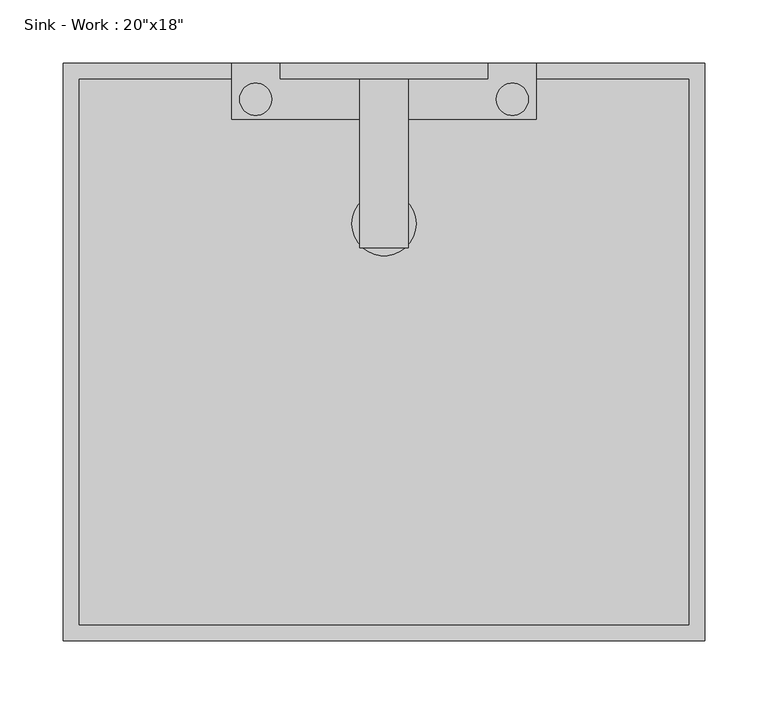
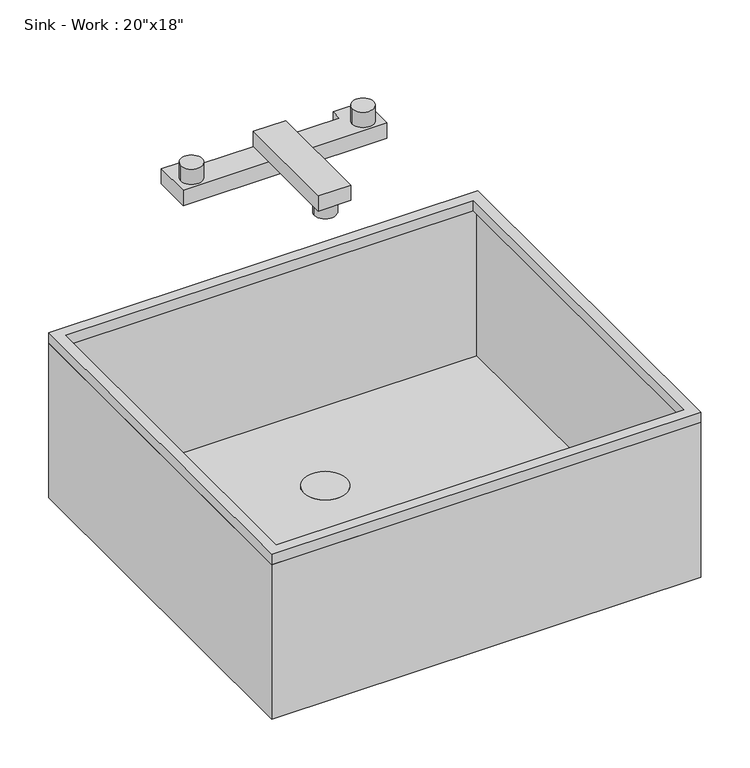
"""IFC4 building model written with IfcOpenShell, lengths in millimetres: flow terminal geometry."""

from ifc_helpers import new_model, si_unit, point, frame, frame_2d, origin, origin_with_axes, place, context, project, spatial, polyline, circle_curve, trimmed, segment, composite_curve, outline, extrude, faceted_brep, source, transform, mapped, element, save
from ifc_brep_helpers import plane_surface, cylinder_surface, advanced_brep


def flow_terminal_98dee406(model_context):
    return source(origin(), model_context, "Body", "SolidModel", [
        extrude(outline(polyline([(254.0, 0.0), (254.0, -457.2), (-254.0, -457.2), (-254.0, 0.0), (254.0, 0.0)]), holes=[polyline([(241.3, -12.7), (-241.3, -12.7), (-241.3, -444.5), (241.3, -444.5), (241.3, -12.7)])]), frame((0.0, 0.0, 193.675), z_axis=(0.0, 0.0, 1.0), x_axis=(1.0, 0.0, 0.0)), (0.0, 0.0, 1.0), 12.7),
        extrude(outline(composite_curve([segment(trimmed(circle_curve(frame_2d((0.0, -127.0)), 25.4), [point((-25.4, -127.0))], [point((25.4, -127.0))], False, "CARTESIAN"), True, "CONTINUOUS"), segment(trimmed(circle_curve(frame_2d((0.0, -127.0)), 25.4), [point((25.4, -127.0))], [point((-25.4, -127.0))], False, "CARTESIAN"), True, "CONTINUOUS")], self_intersect=False)), origin_with_axes(), (0.0, 0.0, 1.0), 3.175),
        faceted_brep([(254.0, 0.0, 193.675), (-254.0, 0.0, 193.675), (-254.0, -457.2, 193.675), (254.0, -457.2, 193.675), (250.825, -3.175, 193.675), (250.825, -454.025, 193.675), (-250.825, -454.025, 193.675), (-250.825, -3.175, 193.675), (254.0, 0.0, 0.0), (254.0, -457.2, 0.0), (-254.0, -457.2, 0.0), (-254.0, 0.0, 0.0), (250.825, -3.175, 3.175), (250.825, -454.025, 3.175), (-250.825, -454.025, 3.175), (-250.825, -3.175, 3.175)], [[[0, 1, 2, 3], [4, 5, 6, 7]], [[8, 9, 10, 11]], [[1, 0, 8, 11]], [[2, 1, 11, 10]], [[3, 2, 10, 9]], [[0, 3, 9, 8]], [[5, 4, 12, 13]], [[6, 5, 13, 14]], [[7, 6, 14, 15]], [[4, 7, 15, 12]], [[13, 12, 15, 14]]]),
        advanced_brep(
        [(19.05, -12.7, 384.175), (-19.05, -12.7, 384.175), (-19.05, -146.05, 384.175), (19.05, -146.05, 384.175), (19.05, -146.05, 365.125), (-19.05, -146.05, 365.125), (-19.05, -44.45, 365.125), (19.05, -44.45, 365.125), (-12.7, -127.0, 365.125), (12.7, -127.0, 365.125), (19.05, -12.7, 365.125), (82.55, -12.7, 365.125), (82.55, -12.7, 346.075), (-82.55, -12.7, 346.075), (-82.55, -12.7, 365.125), (-19.05, -12.7, 365.125), (-12.7, -127.0, 346.075), (12.7, -127.0, 346.075), (-82.55, 0.0, 365.125), (-120.65, 0.0, 365.125), (-120.65, -44.45, 365.125), (-88.9, -28.575, 365.125), (-114.3, -28.575, 365.125), (120.65, -44.45, 365.125), (120.65, 0.0, 365.125), (82.55, 0.0, 365.125), (114.3, -28.575, 365.125), (88.9, -28.575, 365.125), (-82.55, 0.0, 346.075), (82.55, 0.0, 346.075), (120.65, 0.0, 346.075), (120.65, -44.45, 346.075), (-120.65, -44.45, 346.075), (-120.65, 0.0, 346.075), (-114.3, -28.575, 384.175), (-88.9, -28.575, 384.175), (88.9, -28.575, 384.175), (114.3, -28.575, 384.175)],
        [
            (0, 1),
            (1, 2),
            (2, 3),
            (3, 0),
            (4, 5),
            (5, 6),
            (6, 7),
            (7, 4),
            (8, 9, circle_curve(frame((0.0, -127.0, 365.125), z_axis=(0.0, 0.0, 1.0), x_axis=(1.0, 0.0, 0.0)), 12.7)),
            (9, 8, circle_curve(frame((0.0, -127.0, 365.125), z_axis=(0.0, 0.0, 1.0), x_axis=(1.0, 0.0, 0.0)), 12.7)),
            (0, 10),
            (10, 11),
            (11, 12),
            (12, 13),
            (13, 14),
            (14, 15),
            (15, 1),
            (15, 6),
            (5, 2),
            (4, 3),
            (7, 10),
            (16, 17, circle_curve(frame((0.0, -127.0, 346.075), z_axis=(0.0, 0.0, -1.0), x_axis=(1.0, 0.0, 0.0)), 12.7)),
            (17, 16, circle_curve(frame((0.0, -127.0, 346.075), z_axis=(0.0, 0.0, -1.0), x_axis=(1.0, 0.0, 0.0)), 12.7)),
            (17, 9),
            (8, 16),
            (18, 19),
            (19, 20),
            (20, 6),
            (14, 18),
            (21, 22, circle_curve(frame((-101.6, -28.575, 365.125), z_axis=(0.0, 0.0, -1.0), x_axis=(1.0, 0.0, 0.0)), 12.7)),
            (22, 21, circle_curve(frame((-101.6, -28.575, 365.125), z_axis=(0.0, 0.0, -1.0), x_axis=(1.0, 0.0, 0.0)), 12.7)),
            (23, 24),
            (24, 25),
            (25, 11),
            (7, 23),
            (26, 27, circle_curve(frame((101.6, -28.575, 365.125), z_axis=(0.0, 0.0, -1.0), x_axis=(1.0, 0.0, 0.0)), 12.7)),
            (27, 26, circle_curve(frame((101.6, -28.575, 365.125), z_axis=(0.0, 0.0, -1.0), x_axis=(1.0, 0.0, 0.0)), 12.7)),
            (28, 13),
            (12, 29),
            (29, 30),
            (30, 31),
            (31, 32),
            (32, 33),
            (33, 28),
            (18, 28),
            (33, 19),
            (32, 20),
            (31, 23),
            (30, 24),
            (29, 25),
            (34, 35, circle_curve(frame((-101.6, -28.575, 384.175), z_axis=(0.0, 0.0, 1.0), x_axis=(1.0, 0.0, 0.0)), 12.7)),
            (35, 34, circle_curve(frame((-101.6, -28.575, 384.175), z_axis=(0.0, 0.0, 1.0), x_axis=(1.0, 0.0, 0.0)), 12.7)),
            (36, 37, circle_curve(frame((101.6, -28.575, 384.175), z_axis=(0.0, 0.0, 1.0), x_axis=(1.0, 0.0, 0.0)), 12.7)),
            (37, 36, circle_curve(frame((101.6, -28.575, 384.175), z_axis=(0.0, 0.0, 1.0), x_axis=(1.0, 0.0, 0.0)), 12.7)),
            (34, 22),
            (21, 35),
            (36, 27),
            (26, 37),
        ],
        [
            plane_surface(frame((-19.05, -12.7, 384.175), z_axis=(0.0, 0.0, 1.0), x_axis=(-1.0, 0.0, 0.0))),
            plane_surface(frame((-19.05, -12.7, 365.125), z_axis=(0.0, 0.0, -1.0), x_axis=(1.0, 0.0, 0.0))),
            plane_surface(frame((19.05, -12.7, 384.175), z_axis=(0.0, 1.0, 0.0), x_axis=(0.0, 0.0, -1.0))),
            plane_surface(frame((-19.05, -12.7, 384.175), z_axis=(-1.0, 0.0, 0.0), x_axis=(0.0, 0.0, -1.0))),
            plane_surface(frame((-19.05, -146.05, 384.175), z_axis=(0.0, -1.0, 0.0), x_axis=(0.0, 0.0, -1.0))),
            plane_surface(frame((19.05, -146.05, 384.175), z_axis=(1.0, 0.0, 0.0), x_axis=(0.0, 0.0, -1.0))),
            plane_surface(frame((12.7, -127.0, 346.075), z_axis=(0.0, 0.0, -1.0), x_axis=(0.0, -1.0, 0.0))),
            cylinder_surface(frame((0.0, -127.0, 346.075), z_axis=(0.0, 0.0, 1.0), x_axis=(1.0, 0.0, 0.0)), 12.7),
            plane_surface(frame((-120.65, 0.0, 365.125), z_axis=(0.0, 0.0, 1.0), x_axis=(-1.0, 0.0, 0.0))),
            plane_surface(frame((-120.65, 0.0, 346.075), z_axis=(0.0, 0.0, -1.0), x_axis=(1.0, 0.0, 0.0))),
            plane_surface(frame((-82.55, 0.0, 365.125), z_axis=(0.0, 1.0, 0.0), x_axis=(0.0, 0.0, -1.0))),
            plane_surface(frame((-120.65, 0.0, 365.125), z_axis=(-1.0, 0.0, 0.0), x_axis=(0.0, 0.0, -1.0))),
            plane_surface(frame((-120.65, -44.45, 365.125), z_axis=(0.0, -1.0, 0.0), x_axis=(0.0, 0.0, -1.0))),
            plane_surface(frame((120.65, -44.45, 365.125), z_axis=(1.0, 0.0, 0.0), x_axis=(0.0, 0.0, -1.0))),
            plane_surface(frame((120.65, 0.0, 365.125), z_axis=(0.0, 1.0, 0.0), x_axis=(0.0, 0.0, -1.0))),
            plane_surface(frame((82.55, 0.0, 365.125), z_axis=(-1.0, 0.0, 0.0), x_axis=(0.0, 0.0, -1.0))),
            plane_surface(frame((-82.55, -12.7, 365.125), z_axis=(1.0, 0.0, 0.0), x_axis=(0.0, 0.0, -1.0))),
            plane_surface(frame((-88.9, -28.575, 384.175), z_axis=(0.0, 0.0, 1.0), x_axis=(0.0, 1.0, 0.0))),
            cylinder_surface(frame((-101.6, -28.575, 365.125), z_axis=(0.0, 0.0, 1.0), x_axis=(1.0, 0.0, 0.0)), 12.7),
            cylinder_surface(frame((101.6, -28.575, 0.0), z_axis=(0.0, 0.0, 1.0), x_axis=(1.0, 0.0, 0.0)), 12.7),
        ],
        [
            (0, [[1, 2, 3, 4]]),
            (1, [[5, 6, 7, 8], [9, 10]]),
            (2, [[-1, 11, 12, 13, 14, 15, 16, 17]]),
            (3, [[-2, -17, 18, -6, 19]]),
            (4, [[-3, -19, -5, 20]]),
            (5, [[-4, -20, -8, 21, -11]]),
            (6, [[22, 23]]),
            (7, [[-23, 24, -9, 25]]),
            (7, [[-22, -25, -10, -24]]),
            (8, [[26, 27, 28, -18, -16, 29], [30, 31]]),
            (8, [[32, 33, 34, -12, -21, 35], [36, 37]]),
            (9, [[38, -14, 39, 40, 41, 42, 43, 44]]),
            (10, [[-26, 45, -44, 46]]),
            (11, [[-27, -46, -43, 47]]),
            (12, [[-42, 48, -35, -7, -28, -47]]),
            (13, [[-32, -48, -41, 49]]),
            (14, [[-33, -49, -40, 50]]),
            (15, [[-34, -50, -39, -13]]),
            (16, [[-29, -15, -38, -45]]),
            (17, [[51, 52]]),
            (17, [[53, 54]]),
            (18, [[-51, 55, -30, 56]]),
            (18, [[-52, -56, -31, -55]]),
            (19, [[-53, 57, -36, 58]]),
            (19, [[-54, -58, -37, -57]]),
        ],
    ),
    ])


if __name__ == "__main__":
    model = new_model("IFC4")
    model_context = context("Model", 3, world=origin())
    ifc_project = project(units=[si_unit("LENGTHUNIT", "METRE", prefix="MILLI")], contexts=[model_context])
    site = spatial("IfcSite", under=ifc_project)
    building = spatial("IfcBuilding", under=site)
    placement = place(None, origin())
    flow_terminal_shape = flow_terminal_98dee406(model_context)
    element("IfcFlowTerminal", 1, ObjectType="Sink - Work : 20\"x18\"", at=placement, inside=building, context=model_context, shape_type="MappedRepresentation", body=[
        mapped(flow_terminal_shape, transform((0.0, 0.0, 0.0), x_axis=(1.0, 0.0, 0.0), y_axis=(0.0, 1.0, 0.0), z_axis=(0.0, 0.0, 1.0))),
    ])
    save(model, "model.ifc")

# Revit data of these elements
# Type "Sink - Work : 20\"x18\""
#   WFU = 2
#   Sink Width = 1' - 6"
#   Sink Length = 1' - 8"
#   Sink Depth = 0' - 8"
#   Sanitary Radius = 3/4"
#   Sanitary Diameter = 1 1/2"
#   Hot Water Radius = 1/4"
#   Hot Water Diameter = 1/2"
#   HWFU = 2.25
#   Flow Pressure [instance default] = 8.00 psi
#   Faucet Height = 1' - 1 5/8"
#   Cold Water Radius = 1/4"
#   Cold Water Diameter = 1/2"
#   CWFU = 2.25
#   Sink Material = none
#   Faucet Material = none
#   Default Elevation = 0
